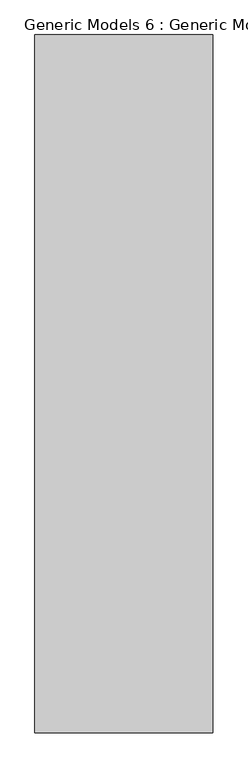
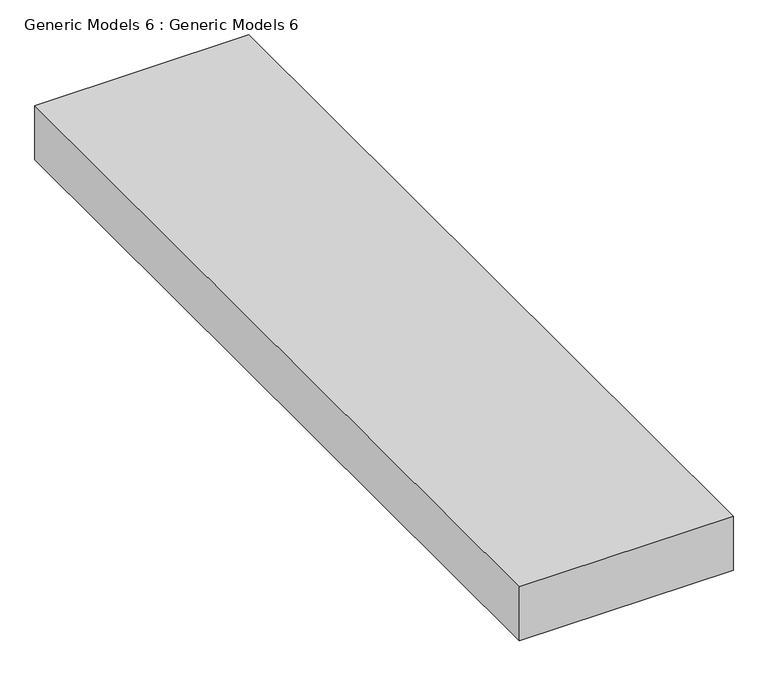
"""IFC4 building model written with IfcOpenShell, lengths in millimetres: proxy geometry, Generic Models 6 : Generic Models 6."""

from ifc_helpers import new_model, si_unit, frame, origin, place, context, project, spatial, polyline, outline, extrude, source, transform, mapped, element, save


def generic_models_6_generic_models_6_d29c9edd(model_context):
    return source(origin(), model_context, "Body", "SweptSolid", [
        extrude(outline(polyline([(-8624.9161422, -12855.0829222), (-9196.4161422, -12855.0829222), (-9196.4161422, -10611.6171312), (-8624.9161422, -10611.6171312), (-8624.9161422, -12855.0829222)])), frame((0.0, 0.0, 2505.560435), z_axis=(0.0, 0.0, 1.0), x_axis=(1.0, 0.0, 0.0)), (0.0, 0.0, 1.0), 152.4),
    ])


if __name__ == "__main__":
    model = new_model("IFC4")
    model_context = context("Model", 3, world=origin())
    ifc_project = project(units=[si_unit("LENGTHUNIT", "METRE", prefix="MILLI")], contexts=[model_context])
    site = spatial("IfcSite", under=ifc_project)
    building = spatial("IfcBuilding", under=site)
    placement = place(None, origin())
    generic_models_6_generic_models_6_shape = generic_models_6_generic_models_6_d29c9edd(model_context)
    element("IfcBuildingElementProxy", 1, Name="Generic Models 6 : Generic Models 6", ObjectType="Generic Models 6 : Generic Models 6", at=placement, inside=building, context=model_context, shape_type="MappedRepresentation", body=[
        mapped(generic_models_6_generic_models_6_shape, transform((0.0, 0.0, 0.0), x_axis=(1.0, 0.0, 0.0), y_axis=(0.0, 1.0, 0.0), z_axis=(0.0, 0.0, 1.0))),
    ])
    save(model, "model.ifc")
